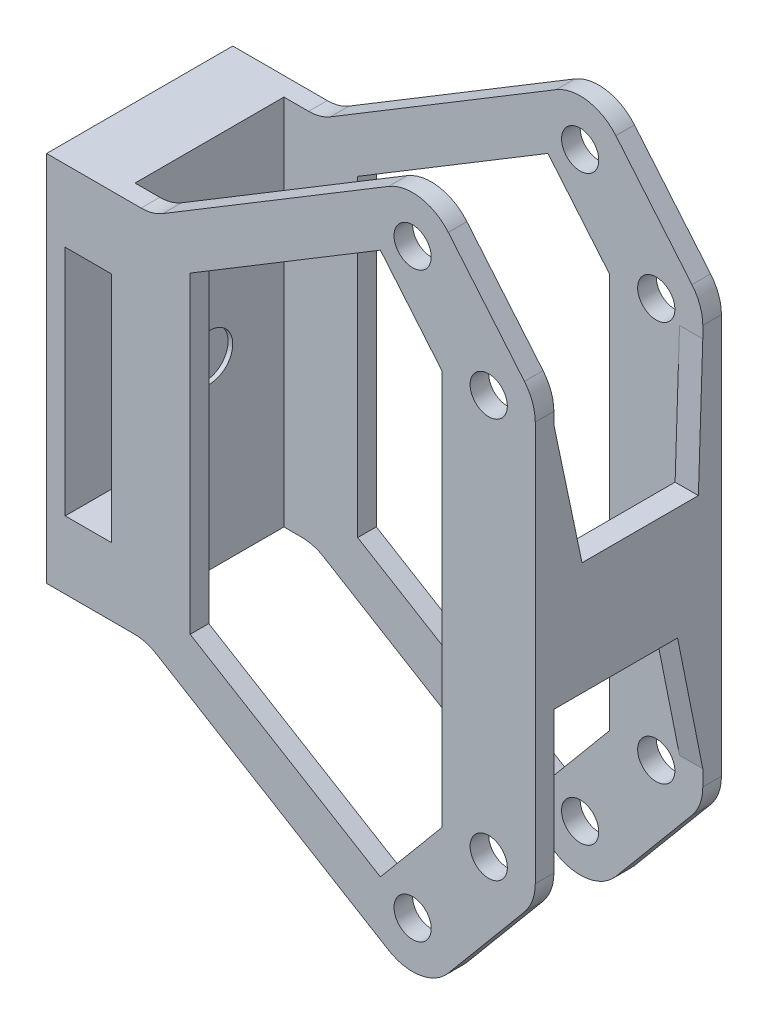
SolidWorks part; units mm, degrees
material "Plain Carbon Steel"
ref_plane "Front Plane" through (0, 0, 0) normal (0, 0, 1) x (1, 0, 0)
ref_plane "Top Plane" through (0, 0, 0) normal (0, 1, 0) x (1, 0, 0)
ref_plane "Right Plane" through (0, 0, 0) normal (1, 0, 0) x (0, 0, -1)
sketch "Bracket Profile Sketch" plane through (0, 0, 0) normal (0, 0, 1) x (1, 0, 0)
  line L0 (18.1127, 41.7389) -> (66.6241, 71.0583)
  line L1 (11.9966, -39.5586) -> (-6.8534, -39.5586)
  line L3 (13.4575, 40.4414) -> (-6.8534, 40.4414)
  line L4 (-6.8534, -39.5586) -> (-6.8534, 40.4414)
  line L11 (7.1466, -25) -> (-2.8534, -25)
  line L12 (7.1466, -25) -> (7.1466, 25)
  line L13 (7.1466, 25) -> (-2.8534, 25)
  line L14 (-2.8534, -25) -> (-2.8534, 25)
  line L15 (7.1466, -25) -> (-2.8534, 25) construction
  line L16 (7.1466, 25) -> (-2.8534, -25) construction
  line L17 (79.4676, 68.9153) -> (95.8176, 49.3653)
  line L18 (98.1466, 42.95) -> (98.1466, -42.95)
  line L21 (23.9966, 33.6106) -> (23.9966, -33.6106)
  line L24 (78.1466, -42.4371) -> (78.1466, 42.4371)
  line L25 (78.1466, 42.4371) -> (64.8692, 58.3132)
  line L26 (64.8692, 58.3132) -> (23.9966, 33.6106)
  line L27 (-52.91, 0) -> (135.4428, 0) construction
  line L28 (79.4676, -68.9153) -> (95.8176, -49.3653)
  line L29 (78.1466, -42.4371) -> (64.8692, -58.3132)
  line L30 (16.6519, -40.856) -> (66.6241, -71.0583)
  line L31 (64.8692, -58.3132) -> (23.9966, -33.6106)
  arc A0 (18.1127, 41.7389) -> (13.4575, 40.4414) centre (13.4575, 49.4414) cw
  arc A1 (11.9966, -39.5586) -> (16.6519, -40.856) centre (11.9966, -48.5586) cw
  arc A4 (95.8176, 49.3653) -> (98.1466, 42.95) centre (88.1466, 42.95) cw
  arc A5 (66.6241, 71.0583) -> (79.4676, 68.9153) centre (71.7966, 62.5) cw
  circle A8 centre (88.1466, 42.95) radius 4
  circle A9 centre (71.7966, 62.5) radius 4
  arc A10 (95.8176, -49.3653) -> (98.1466, -42.95) centre (88.1466, -42.95) ccw
  circle A11 centre (88.1466, -42.95) radius 4
  circle A12 centre (71.7966, -62.5) radius 4
  arc A13 (66.6241, -71.0583) -> (79.4676, -68.9153) centre (71.7966, -62.5) ccw
  point P0 (0, 0)
  point P6 (0, 0)
  point P7 (2.1466, 0)
  point P24 (98.1466, 0)
  point P31 (78.1466, 0)
  point P48 (23.9966, 0)
  dimension "D12" = 9
  dimension "D13" = 54.15
  dimension "D14" = 42.95
  dimension "D18" = 8
  dimension "D1" = 80
  dimension "D2" = 4.85
  dimension "D3" = 4
  dimension "D4" = 10
  dimension "D5" = 50
  dimension "D6" = 25
  dimension "D8" = 16.35
  dimension "D7" = 10
  dimension "D9" = 19.55
  dimension "D10" = 18
  dimension "D11" = 20
  dimension "D15" = 10
  dimension "D16" = 105
  dimension "D17" = 11.9966
  dimension "D19" = 49.4414
extrude "Bracket Body" add sketch "Bracket Profile Sketch" along normal mid plane 40
sketch "Side Cutout Sketch" plane through (0, 40.4414, 0) normal (0, 1, 0) x (1, 0, 0)
  line L5 (98.1466, -20) -> (98.1466, 20) construction
  line L6 (93.1466, -16) -> (8.1466, -16)
  line L8 (93.1466, -16) -> (93.1466, 16)
  line L9 (93.1466, 16) -> (8.1466, 16)
  line L10 (8.1466, -16) -> (8.1466, 16)
  line L11 (93.1466, -16) -> (8.1466, 16) construction
  line L12 (93.1466, 16) -> (8.1466, -16) construction
  point P0 (50.6466, 0)
  dimension "D1" = 85
  dimension "D2" = 5
  dimension "D3" = 32
extrude "Side Cutout" cut sketch "Side Cutout Sketch" against normal through all both and the other way through all
sketch "Inner Window Sketch" plane through (-6.8534, 0, 0) normal (-1, 0, 0) x (0, 0, 1)
  line L0 (-16, 40.4414) -> (16, 40.4414)
  line L1 (20, 40.4414) -> (-20, 40.4414) construction
  line L2 (-16, -39.5586) -> (16, -39.5586)
  line L3 (-16, -39.5586) -> (-20, -39.5586) construction
  line L4 (16, -52.559) -> (16, 52.559)
  line L5 (16, 52.559) -> (-16, 52.559)
  line L6 (-16, 52.559) -> (-16, -52.559)
  line L7 (-16, -52.559) -> (16, -52.559)
  line L8 (16, -52.559) -> (16, -39.5586)
  line L9 (16, 52.559) -> (-16, 52.559)
  line L10 (-16, 52.559) -> (-16, 40.4414)
  line L11 (-16, -52.559) -> (16, -52.559)
  line L12 (20, -39.5586) -> (-20, -39.5586) construction
  line L13 (-16, -39.5586) -> (-16, -52.559)
  line L14 (16, 40.4414) -> (16, 52.559)
  dimension "D1" = 0
extrude "Inner Window Cut" cut sketch "Inner Window Sketch" against normal through all both
sketch "Side Openings Sketch" plane through (98.1466, 0, 0) normal (1, 0, 0) x (0, 0, -1)
  line L0 (-16, -39.5586) -> (-16, -12.5)
  line L5 (-16, 40.4414) -> (-9.9509, 11.7571)
  line L6 (-16, -12.5) -> (10.5796, -12.5)
  line L8 (-9.9509, 11.7571) -> (15.0491, 11.7571)
  line L10 (-16, -12.5) -> (15.0491, 11.7571) construction
  line L11 (-9.9509, 11.7571) -> (10.5796, -12.5) construction
  line L12 (16, 40.4414) -> (15.0491, 11.7571)
  line L13 (16, -39.5586) -> (10.5796, -12.5)
  line L23 (-16, -39.5586) -> (16, -39.5586)
  line L24 (16, -39.5586) -> (16, -42.95)
  line L25 (16, -42.95) -> (20, -42.95)
  line L26 (20, -42.95) -> (20, 42.95)
  line L27 (20, 42.95) -> (16, 42.95)
  line L28 (16, 42.95) -> (16, 40.4414)
  line L29 (16, 40.4414) -> (-16, 40.4414)
  line L30 (-16, 40.4414) -> (-16, 42.95)
  line L31 (-16, 42.95) -> (-20, 42.95)
  line L32 (-20, 42.95) -> (-20, -42.95)
  line L33 (-20, -42.95) -> (-16, -42.95)
  line L34 (-16, -42.95) -> (-16, -39.5586)
  line L35 (-16, -39.5586) -> (16, -39.5586)
  line L41 (16, 40.4414) -> (-16, 40.4414)
  point P0 (0, 0)
  dimension "D1" = 25
  dimension "D2" = 25
  dimension "D4" = 12.5
  dimension "D5" = 27.0586
  dimension "D3" = 0
extrude "Side Openings Cut" cut sketch "Side Openings Sketch" against normal blind 40
sketch "Hole Ø10 Sketch" plane through (-6.8534, 0, 0) normal (-1, 0, 0) x (0, 0, 1)
  circle A0 centre (0, 0) radius 5
  dimension "D1" = 10
extrude "Through Hole Ø10" cut sketch "Hole Ø10 Sketch" against normal blind 40
sketch "Recess Ø24 Sketch" plane through (-6.8534, 0, 0) normal (-1, 0, 0) x (0, 0, 1)
  circle A0 centre (0, 0) radius 12
  dimension "D1" = 24
extrude "Recess Ø24x3" cut sketch "Recess Ø24 Sketch" against normal blind 3
